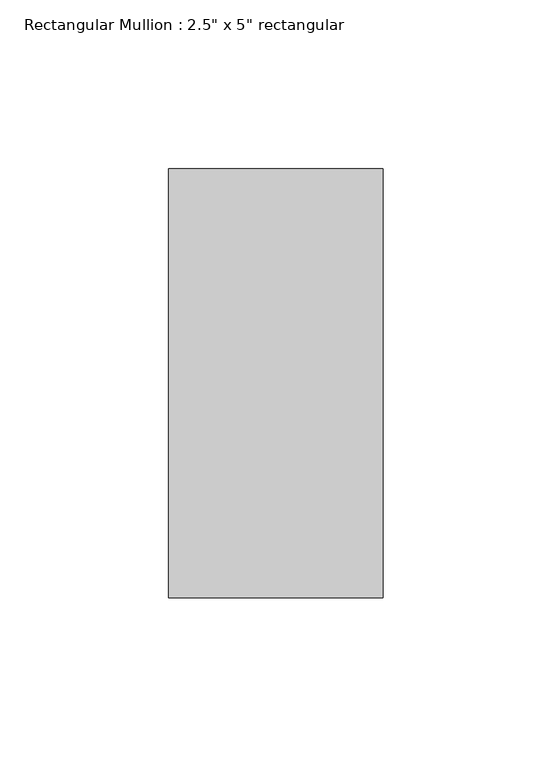
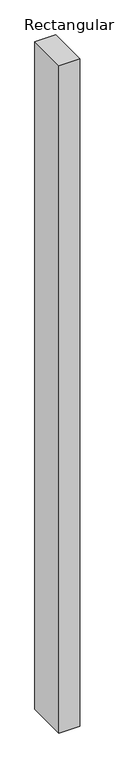
"""IFC4 building model written with IfcOpenShell, lengths in millimetres: member geometry."""

from ifc_helpers import new_model, si_unit, frame, origin, place, context, project, spatial, polyline, outline, extrude, source, transform, mapped, element, save


def member_c08f7e50(model_context):
    return source(origin(), model_context, "Body", "SweptSolid", [
        extrude(outline(polyline([(0.0, 63.5), (0.0, -63.5), (-63.5, -63.5), (-63.5, 63.5), (0.0, 63.5)])), frame((0.0, 0.0, -2159.0), z_axis=(0.0, 0.0, 1.0), x_axis=(1.0, 0.0, 0.0)), (0.0, 0.0, 1.0), 2159.0),
    ])


if __name__ == "__main__":
    model = new_model("IFC4")
    model_context = context("Model", 3, world=origin())
    ifc_project = project(units=[si_unit("LENGTHUNIT", "METRE", prefix="MILLI")], contexts=[model_context])
    site = spatial("IfcSite", under=ifc_project)
    building = spatial("IfcBuilding", under=site)
    placement = place(None, origin())
    member_shape = member_c08f7e50(model_context)
    element("IfcMember", 1, ObjectType="Rectangular Mullion : 2.5\" x 5\" rectangular", at=placement, inside=building, context=model_context, shape_type="MappedRepresentation", body=[
        mapped(member_shape, transform((0.0, 0.0, 0.0), x_axis=(1.0, 0.0, 0.0), y_axis=(0.0, 1.0, 0.0), z_axis=(0.0, 0.0, 1.0))),
    ])
    save(model, "model.ifc")

# Revit data of these elements
# Type "Rectangular Mullion : 2.5\" x 5\" rectangular"
#   built-in parameter 1007304 = 0.416667 (stored number, unit not read)
#   built-in parameter 1007301 = 0.104167 (stored number, unit not read)
#   built-in parameter 1007300 = 0.104167 (stored number, unit not read)
